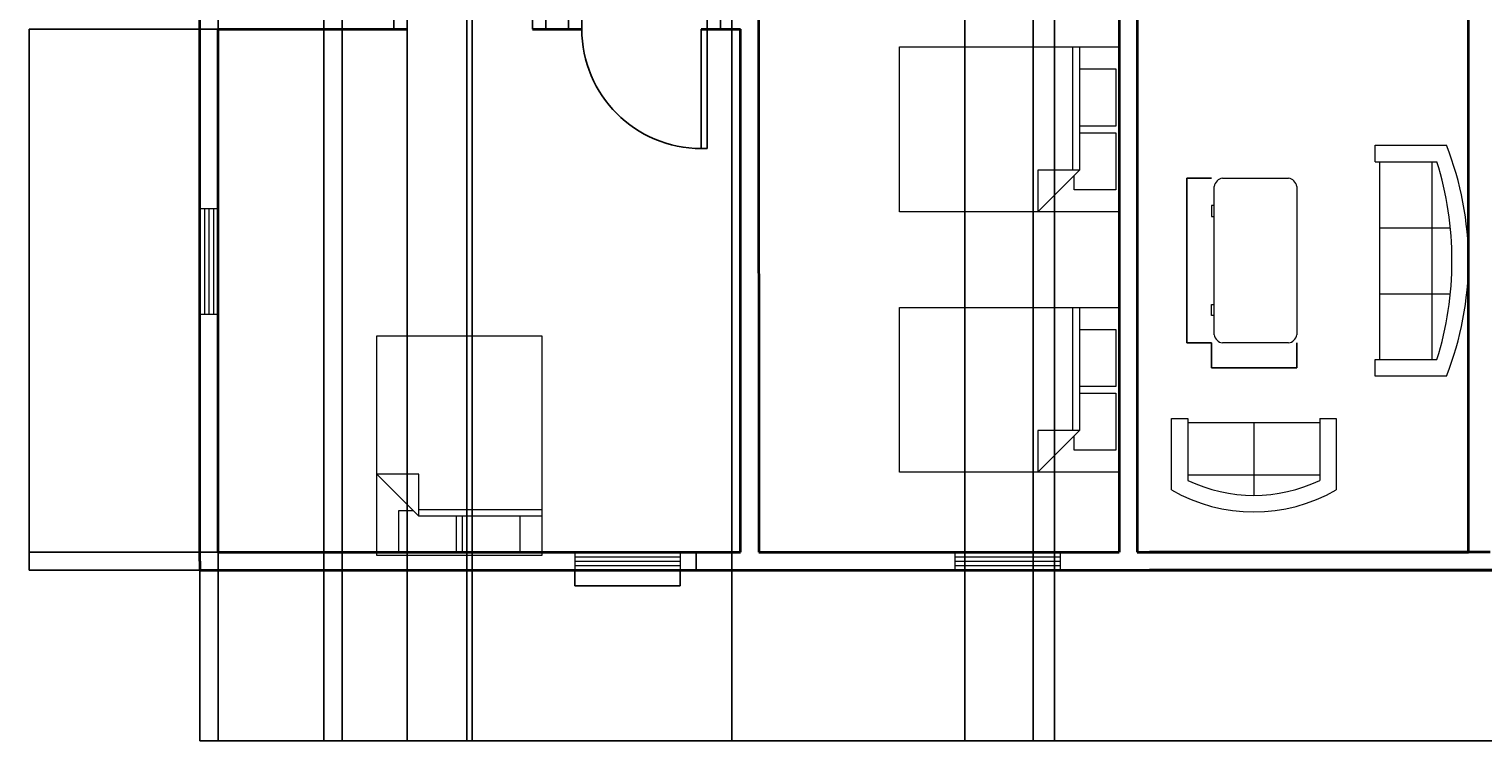
# Model space of a CAD drawing. Units: millimetres. Extents: x 31 to 27050, y -916 to 32407.
# Tile 1 of 7: x 31 to 13474, y -916 to 5664. Entities that reach past the tile are written whole.
import ezdxf

# ---------------------------------------------------------------- set-up
doc = ezdxf.new("R2010")
doc.units = ezdxf.units.MM
for name, color, linetype, lineweight in [('A-ANNO-DIMS', 2, 'Continuous', 18), ('A-DOOR', 3, 'Continuous', 25), ('A-FURN', 8, 'Continuous', 13), ('A-GLAZ', 4, 'Continuous', 18), ('A-WALL', 7, 'Continuous', 35)]:
    doc.layers.add(name, color=color, linetype=linetype, lineweight=lineweight)
doc.styles.get("Standard").update_dxf_attribs({"font": 'arial.ttf'})
doc.dimstyles.get("Standard").update_dxf_attribs({"dimtxt": 0.18, "dimasz": 0.18, "dimexe": 0.18, "dimexo": 0.0625, "dimgap": 0.09, "dimtad": 0, "dimtih": 1, "dimtoh": 1, "dimdec": 4, "dimzin": 0, "dimdsep": 46, "dimtxsty": 'Standard', "dimcen": 0.09, "dimadec": 0, "dimazin": 0, "dimtfac": 1, "dimtdec": 4, "dimtofl": 0, "dimtmove": 0, "dimatfit": 3, "dimfxl": 1, "dimtolj": 1, "dimtzin": 0, "dimarcsym": 0})

# ---------------------------------------------------------------- blocks, each defined once
blk = doc.blocks.new('Sofa - Roundback 7 ft.')
for p, q in [((-12.00002, -32.44210000000393), (-12.00003, -6.597100000003898)), ((11.99996999999999, -32.44210000000393), (11.99997999999999, -6.597100000003898)), ((-36.000027, -34.00000000000395), (-36.000027, -11.46960000000396)), ((-35.999844, -13.38190000000397), (35.99979999999999, -13.38190000000397)), ((35.99997999999999, -34.00000000000395), (35.99997999999999, -11.46960000000396)), ((-36.000027, -32.44210000000393), (35.99997999999999, -32.44210000000393))]:
    blk.add_line(p, q)
for points in [[(-36.000027, -34.00000000000395), (-42.000027, -34.00000000000395), (-42.000027, -8.000000000003944)], [(41.99997999999999, -8.000000000003944), (41.99997999999999, -34.00000000000395), (35.99997999999999, -34.00000000000395)]]:
    blk.add_lwpolyline(points)
for centre, radius, start, end in [((0, -114.2500000000039), 114.2500000000039, 68.43141000000072, 111.5686000000006), ((-1.00000000032e-05, -127.1968000000039), 121.1967999999973, 72.72032999999948, 107.2797000000005)]:
    blk.add_arc(centre, radius, start, end)
blk = doc.blocks.new('Sofa - Roundback Loveseat 5 ft.')
for p, q in [((0, -32.44198000000246), (0, -5.999980000002448)), ((-23.99999999999999, -33.99998000000245), (-23.99999999999999, -11.46958000000243)), ((-23.99979999999998, -13.38178000000245), (23.99986, -13.38178000000245)), ((24.00004000000001, -33.99998000000245), (24.00004000000001, -11.46958000000243)), ((-23.99999999999999, -32.44198000000246), (24.00004000000001, -32.44198000000246))]:
    blk.add_line(p, q)
for points in [[(-23.99999999999999, -33.99998000000245), (-29.99999999999999, -33.99998000000245), (-29.99999999999999, -7.999980000002448)], [(30.00004000000001, -7.999980000002448), (30.00004000000001, -33.99998000000245), (24.00004000000001, -33.99998000000245)]]:
    blk.add_lwpolyline(points)
for centre, radius, start, end in [((0, -60.24998000000245), 60.24998000000245, 60.13715000000122, 119.862800000004), ((0, -61.38438000000245), 55.38444000000723, 64.32083000000306, 115.6791999999996)]:
    blk.add_arc(centre, radius, start, end)
blk = doc.blocks.new('Desk - 30 x 60 in.')
for p, q in [((-26.999995, 0), (26.999995, 0)), ((-29.999995, -27), (-29.999995, -3)), ((29.999995, -3), (29.999995, -27)), ((26.999995, -30), (-26.999995, -30)), ((-20.000005, -30), (-20.000005, -31)), ((-20.000005, -31), (-16.000005, -31)), ((-16.000005, -31), (-16.000005, -30)), ((15.999995, -31), (15.999995, -30)), ((19.999995, -31), (15.999995, -31)), ((19.999995, -30), (19.999995, -31))]:
    blk.add_line(p, q)
for centre, radius, start, end in [((-26.499995, -3.5), 3.535534000004229, 98.1300999999916, 171.8698999999352), ((26.499995, -3.5), 3.535533999997753, 8.130102000022115, 81.8698999999439), ((-26.499995, -26.5), 3.535534000000845, 188.1301000000653, 261.8699000000085), ((26.499995, -26.5), 3.535534000004826, 278.1301000000561, 351.8698999999439)]:
    blk.add_arc(centre, radius, start, end)
blk = doc.blocks.new('Bed - Queen')
for p, q in [((0, -80.00003000000002), (0, 0)), ((0, 0), (59.99998999999999, 0)), ((59.99998999999999, 0), (59.99998999999999, -80.00003000000002)), ((7.99999, -1.200000000000017), (28.79998, -1.200000000000017)), ((7.99999, -14.4), (7.99999, -1.200000000000017)), ((28.79998, -1.200000000000017), (28.79998, -14.4)), ((31.19999, -1.200000000000017), (51.99999000000001, -1.200000000000017)), ((31.19999, -14.4), (31.19999, -1.200000000000017)), ((51.99999000000001, -1.200000000000017), (51.99999000000001, -16.4)), ((0, -14.4), (44.79999999999999, -14.4)), ((59.99998999999999, -29.60000000000001), (44.79999999999999, -14.4)), ((44.79999999999999, -14.4), (44.79999999999999, -29.60000000000001)), ((44.79999999999999, -16.80000000000001), (0, -16.80000000000001)), ((51.99999000000001, -16.4), (46.79936, -16.4)), ((44.79999999999999, -29.60000000000001), (59.99998999999999, -29.60000000000001)), ((59.99998999999999, -80.00003000000002), (0, -80.00003000000002))]:
    blk.add_line(p, q)
blk = doc.blocks.new('Window - Wood Frame 36 in. Wide plan')
for p, q in [((0, 6), (0, 0)), ((36, 6), (36, 0)), ((0, 4.5), (36, 4.5)), ((0, 3), (36, 3)), ((0, 1.5), (36, 1.5))]:
    blk.add_line(p, q)
blk = doc.blocks.new('DOOR-SINGLE-1104')
for p, q in [((56.41678681898429, 1104.337341461596), (-7.18501e-11, 1104.337341461596)), ((-7.18501e-11, 1104.337341461596), (-7.18501e-11, 3.638e-12)), ((56.41678681898429, 7.276e-12), (56.41678681898429, 1104.337341461596)), ((-1226.913698425656, -163.8831223050438), (-1226.913698425656, 3.638e-12)), ((-1104.337341461589, 3.638e-12), (-1226.913698425656, 7.276e-12)), ((-1104.337341461589, 3.638e-12), (-1104.337341461589, -163.8831223050438)), ((-7.18501e-11, 3.638e-12), (56.41678681898429, 7.276e-12)), ((56.41678681898429, -163.8831223050438), (56.41678681898429, 3.638e-12)), ((56.41678681898429, 3.638e-12), (178.9931437830519, 3.638e-12)), ((178.9931437830519, 3.638e-12), (178.9931437830519, -163.8831223050438)), ((-1104.337341461589, -163.8831223050438), (-1226.913698425656, -163.8831223050438)), ((178.9931437830519, -163.8831223050438), (56.41678681898429, -163.8831223050438))]:
    blk.add_line(p, q)
blk.add_arc((0, 3.638e-12), 1104.337341461589, 90, 180)
blk = doc.blocks.new('*D20')
at = {"layer": 'A-ANNO-DIMS', "color": 0, "lineweight": -2, "transparency": 16777216}
for p, q in [((5076.661328165442, 664.7949646643646), (5076.661328165442, 518.2710500577334)), ((6052.70409220965, 664.7949646643646), (6052.70409220965, 518.2710500577334)), ((5076.841328165443, 518.4510500577334), (5563.054422329429, 518.4510500577334)), ((6052.52409220965, 518.4510500577334), (5566.310998045663, 518.4510500577334))]:
    blk.add_line(p, q, dxfattribs=at)
at = {"layer": 'A-ANNO-DIMS', "color": 0, "transparency": 16777216}
for points in [[(5076.841328165443, 518.4810500577335), (5076.841328165443, 518.4210500577335), (5076.661328165442, 518.4510500577334)], [(6052.52409220965, 518.4810500577335), (6052.52409220965, 518.4210500577335), (6052.70409220965, 518.4510500577334)]]:
    blk.add_solid(points, dxfattribs=at)
at = {"layer": 'Defpoints', "color": 0, "transparency": 16777216}
for p in [(5076.661328165442, 664.8574646643647), (6052.70409220965, 664.8574646643647), (6052.70409220965, 518.4510500577334)]:
    blk.add_point(p, dxfattribs=at)
at = {"layer": 'A-ANNO-DIMS', "color": 0, "transparency": 16777216, "insert": (5564.682710187546, 518.4510500577334), "char_height": 0.18, "attachment_point": 5}
blk.add_mtext('\\A1;WOOD WINDOW 976 TYP.', dxfattribs=at)
blk = doc.blocks.new('*D21')
at = {"layer": 'A-ANNO-DIMS', "color": 0, "lineweight": -2, "transparency": 16777216}
for p, q in [((6052.766592209652, 827.531258671733), (6199.290506816289, 827.531258671733)), ((6199.110506816289, 827.351258671733), (6199.110506816289, 746.3763261973802)), ((6199.110506816289, 665.0374646643648), (6199.110506816289, 746.0123971387173)), ((6052.766592209652, 664.8574646643648), (6199.290506816289, 664.8574646643648))]:
    blk.add_line(p, q, dxfattribs=at)
at = {"layer": 'A-ANNO-DIMS', "color": 0, "transparency": 16777216}
for points in [[(6199.080506816289, 827.351258671733), (6199.140506816288, 827.351258671733), (6199.110506816289, 827.531258671733)], [(6199.080506816289, 665.0374646643648), (6199.140506816288, 665.0374646643648), (6199.110506816289, 664.8574646643648)]]:
    blk.add_solid(points, dxfattribs=at)
at = {"layer": 'Defpoints', "color": 0, "transparency": 16777216}
for p in [(6052.704092209652, 827.531258671733), (6199.110506816289, 827.531258671733), (6052.704092209652, 664.8574646643648)]:
    blk.add_point(p, dxfattribs=at)
at = {"layer": 'A-ANNO-DIMS', "color": 0, "transparency": 16777216, "insert": (6199.110506816287, 746.194361668047), "char_height": 0.18, "attachment_point": 5}
blk.add_mtext('\\A1;163 TYP.', dxfattribs=at)
blk = doc.blocks.new('*D38')
at = {"layer": 'A-ANNO-DIMS', "color": 0, "lineweight": -2, "transparency": 16777216}
for p, q in [((10964.92577730674, 4286.348550041928), (10736.20831454058, 4286.348550041928)), ((10736.38831454058, 4286.168550041928), (10736.38831454058, 3524.531743731799)), ((10736.38831454058, 2762.528798267508), (10736.38831454058, 3524.165604577638)), ((10964.92577730674, 2762.348798267508), (10736.20831454058, 2762.348798267508))]:
    blk.add_line(p, q, dxfattribs=at)
at = {"layer": 'A-ANNO-DIMS', "color": 0, "transparency": 16777216}
for points in [[(10736.35831454058, 4286.168550041928), (10736.41831454058, 4286.168550041928), (10736.38831454058, 4286.348550041928)], [(10736.35831454058, 2762.528798267508), (10736.41831454058, 2762.528798267508), (10736.38831454058, 2762.348798267508)]]:
    blk.add_solid(points, dxfattribs=at)
at = {"layer": 'Defpoints', "color": 0, "transparency": 16777216}
for p in [(10964.98827730674, 4286.348550041928), (10736.38831454058, 2762.348798267508), (10964.98827730674, 2762.348798267508)]:
    blk.add_point(p, dxfattribs=at)
at = {"layer": 'A-ANNO-DIMS', "color": 0, "transparency": 16777216, "insert": (10736.38831454058, 3524.348674154714), "char_height": 0.18, "attachment_point": 5}
blk.add_mtext('\\A1;DESK 1524 TYP.', dxfattribs=at)
blk = doc.blocks.new('*D39')
at = {"layer": 'A-ANNO-DIMS', "color": 0, "lineweight": -2, "transparency": 16777216}
for p, q in [((10964.98827730674, 2762.286298267507), (10964.98827730674, 2533.568835501344)), ((11752.38828019396, 2762.286298267507), (11752.38828019396, 2533.568835501344)), ((10965.16827730674, 2533.748835501344), (11358.09100044202, 2533.748835501344)), ((11752.20828019396, 2533.748835501344), (11359.28555705867, 2533.748835501344))]:
    blk.add_line(p, q, dxfattribs=at)
at = {"layer": 'A-ANNO-DIMS', "color": 0, "transparency": 16777216}
for points in [[(10965.16827730674, 2533.778835501344), (10965.16827730674, 2533.718835501344), (10964.98827730674, 2533.748835501344)], [(11752.20828019396, 2533.778835501344), (11752.20828019396, 2533.718835501344), (11752.38828019396, 2533.748835501344)]]:
    blk.add_solid(points, dxfattribs=at)
at = {"layer": 'Defpoints', "color": 0, "transparency": 16777216}
for p in [(10964.98827730674, 2762.348798267507), (11752.38828019396, 2762.348798267507), (11752.38828019396, 2533.748835501344)]:
    blk.add_point(p, dxfattribs=at)
at = {"layer": 'A-ANNO-DIMS', "color": 0, "transparency": 16777216, "insert": (11358.68827875035, 2533.748835501344), "char_height": 0.18, "attachment_point": 5}
blk.add_mtext('\\A1;787 TYP.', dxfattribs=at)
blk = doc.blocks.new('*D46')
at = {"layer": 'A-ANNO-DIMS', "color": 0, "lineweight": -2, "transparency": 16777216}
for p, q in [((1610.021997, 663.585636), (1610.021997, -915.531864)), ((25471.148668, 663.585636), (25471.148668, -915.531864)), ((1610.201997, -915.3518639999999), (13540.17247438267, -915.3518639999999)), ((25470.968668, -915.3518639999999), (13540.99819061733, -915.3518639999999))]:
    blk.add_line(p, q, dxfattribs=at)
at = {"layer": 'A-ANNO-DIMS', "color": 0, "transparency": 16777216}
for points in [[(1610.201997, -915.321864), (1610.201997, -915.381864), (1610.021997, -915.3518639999999)], [(25470.968668, -915.321864), (25470.968668, -915.381864), (25471.148668, -915.3518639999999)]]:
    blk.add_solid(points, dxfattribs=at)
at = {"layer": 'Defpoints', "color": 0, "transparency": 16777216}
for p in [(1610.021997, 663.648136), (25471.148668, 663.648136), (25471.148668, -915.3518639999999)]:
    blk.add_point(p, dxfattribs=at)
at = {"layer": 'A-ANNO-DIMS', "color": 0, "transparency": 16777216, "insert": (13540.5853325, -915.3518639999999), "char_height": 0.18, "attachment_point": 5}
blk.add_mtext('\\A1;23861', dxfattribs=at)
blk = doc.blocks.new('*D59')
at = {"layer": 'A-ANNO-DIMS', "color": 0, "lineweight": -2, "transparency": 16777216}
for p, q in [((1778.310148000001, 5663.648136000002), (30.84199699999942, 5663.648136000002)), ((31.02199699999949, 5663.468136000002), (31.02199700000003, 3245.771662029333)), ((31.02199700000057, 827.7112590000002), (31.02199700000003, 3245.407732970669)), ((1778.310148000001, 827.5312590000003), (30.8419970000005, 827.5312590000002))]:
    blk.add_line(p, q, dxfattribs=at)
at = {"layer": 'A-ANNO-DIMS', "color": 0, "transparency": 16777216}
for points in [[(30.99199699999949, 5663.468136000002), (31.05199699999949, 5663.468136000002), (31.02199699999949, 5663.648136000002)], [(30.99199700000057, 827.7112590000002), (31.05199700000057, 827.7112590000002), (31.02199700000057, 827.5312590000002)]]:
    blk.add_solid(points, dxfattribs=at)
at = {"layer": 'Defpoints', "color": 0, "transparency": 16777216}
for p in [(31.02199699999949, 5663.648136000002), (1778.372648000001, 5663.648136000002), (1778.372648000001, 827.5312590000003)]:
    blk.add_point(p, dxfattribs=at)
at = {"layer": 'A-ANNO-DIMS', "color": 0, "transparency": 16777216, "insert": (31.02199700000094, 3245.5896975), "char_height": 0.18, "attachment_point": 5}
blk.add_mtext('\\A1;4836', dxfattribs=at)
blk = doc.blocks.new('*D69')
at = {"layer": 'A-ANNO-DIMS', "color": 0, "lineweight": -2, "transparency": 16777216}
for p, q in [((2757.340836, 14467.362437), (2757.340835999999, -915.5318640000004)), ((4128.594056999999, 14467.362437), (4128.594056999999, -915.5318640000004)), ((2757.520835999999, -915.3518639999999), (3442.512289610504, -915.3518639999999)), ((4128.414056999999, -915.3518639999999), (3443.422603389495, -915.3518639999999))]:
    blk.add_line(p, q, dxfattribs=at)
at = {"layer": 'A-ANNO-DIMS', "color": 0, "transparency": 16777216}
for points in [[(2757.520835999999, -915.321864), (2757.520835999999, -915.381864), (2757.340835999999, -915.3518639999999)], [(4128.414056999999, -915.321864), (4128.414056999999, -915.381864), (4128.594056999999, -915.3518639999999)]]:
    blk.add_solid(points, dxfattribs=at)
at = {"layer": 'Defpoints', "color": 0, "transparency": 16777216}
for p in [(2757.340836, 14467.424937), (4128.594056999999, 14467.424937), (4128.594056999999, -915.3518639999999)]:
    blk.add_point(p, dxfattribs=at)
at = {"layer": 'A-ANNO-DIMS', "color": 0, "transparency": 16777216, "insert": (3442.967446499999, -915.3518639999999), "char_height": 0.18, "attachment_point": 5}
blk.add_mtext('\\A1;1371.3', dxfattribs=at)
blk = doc.blocks.new('*D70')
at = {"layer": 'A-ANNO-DIMS', "color": 0, "lineweight": -2, "transparency": 16777216}
for p, q in [((4128.594056999999, 14467.362437), (4128.594056999999, -915.5318640000004)), ((6528.594057000001, 14467.362437), (6528.594056999999, -915.5318640000004)), ((4128.774057, -915.3518639999999), (5328.234056999999, -915.3518639999999)), ((6528.414056999999, -915.3518639999999), (5328.954056999999, -915.3518639999999))]:
    blk.add_line(p, q, dxfattribs=at)
at = {"layer": 'A-ANNO-DIMS', "color": 0, "transparency": 16777216}
for points in [[(4128.774057, -915.321864), (4128.774057, -915.381864), (4128.594056999999, -915.3518639999999)], [(6528.414056999999, -915.321864), (6528.414056999999, -915.381864), (6528.594056999999, -915.3518639999999)]]:
    blk.add_solid(points, dxfattribs=at)
at = {"layer": 'Defpoints', "color": 0, "transparency": 16777216}
for p in [(4128.594056999999, 14467.424937), (6528.594057000001, 14467.424937), (6528.594056999999, -915.3518639999999)]:
    blk.add_point(p, dxfattribs=at)
at = {"layer": 'A-ANNO-DIMS', "color": 0, "transparency": 16777216, "insert": (5328.594057, -915.3518639999999), "char_height": 0.18, "attachment_point": 5}
blk.add_mtext('\\A1;2400', dxfattribs=at)
blk = doc.blocks.new('*D74')
at = {"layer": 'A-ANNO-DIMS', "color": 0, "lineweight": -2, "transparency": 16777216}
for p, q in [((8684.522829, 19025.373224), (8684.522828999998, -915.5318640000004)), ((9513.331407, 19025.373224), (9513.331407, -915.5318640000004)), ((8684.702829, -915.3518639999999), (9098.533107085947, -915.3518639999999)), ((9513.151406999998, -915.3518639999999), (9099.321128914047, -915.3518639999999))]:
    blk.add_line(p, q, dxfattribs=at)
at = {"layer": 'A-ANNO-DIMS', "color": 0, "transparency": 16777216}
for points in [[(8684.702829, -915.321864), (8684.702829, -915.381864), (8684.522828999998, -915.3518639999999)], [(9513.151406999998, -915.321864), (9513.151406999998, -915.381864), (9513.331407, -915.3518639999999)]]:
    blk.add_solid(points, dxfattribs=at)
at = {"layer": 'Defpoints', "color": 0, "transparency": 16777216}
for p in [(8684.522829, 19025.435724), (9513.331407, 19025.435724), (8684.522828999998, -915.3518639999999)]:
    blk.add_point(p, dxfattribs=at)
at = {"layer": 'A-ANNO-DIMS', "color": 0, "transparency": 16777216, "insert": (9098.927117999998, -915.3518639999999), "char_height": 0.18, "attachment_point": 5}
blk.add_mtext('\\A1;828.8', dxfattribs=at)
blk = doc.blocks.new('*D75')
at = {"layer": 'A-ANNO-DIMS', "color": 0, "lineweight": -2, "transparency": 16777216}
for p, q in [((9315.42813, 12465.681171), (9315.42813, -915.5318640000004)), ((9513.331407, 12465.681171), (9513.331407, -915.5318640000004)), ((9315.60813, -915.3518639999999), (9413.994352401773, -915.3518639999999)), ((9513.151407, -915.3518639999999), (9414.765184598225, -915.3518639999999))]:
    blk.add_line(p, q, dxfattribs=at)
at = {"layer": 'A-ANNO-DIMS', "color": 0, "transparency": 16777216}
for points in [[(9315.60813, -915.321864), (9315.60813, -915.381864), (9315.42813, -915.3518639999999)], [(9513.151407, -915.321864), (9513.151407, -915.381864), (9513.331407, -915.3518639999999)]]:
    blk.add_solid(points, dxfattribs=at)
at = {"layer": 'Defpoints', "color": 0, "transparency": 16777216}
for p in [(9315.42813, 12465.743671), (9513.331407, 12465.743671), (9513.331407, -915.3518639999999)]:
    blk.add_point(p, dxfattribs=at)
at = {"layer": 'A-ANNO-DIMS', "color": 0, "transparency": 16777216, "insert": (9414.379768499999, -915.3518639999999), "char_height": 0.18, "attachment_point": 5}
blk.add_mtext('\\A1;197.9', dxfattribs=at)
blk = doc.blocks.new('*D88')
at = {"layer": 'A-ANNO-DIMS', "color": 0, "lineweight": -2, "transparency": 16777216}
for p, q in [((1778.310148000001, 827.5312590000003), (30.84199700000004, 827.5312590000002)), ((31.02199700000001, 827.3512590000003), (31.02199700000003, 745.7716620293315)), ((31.02199700000005, 663.8281359999999), (31.02199700000003, 745.4077329706685)), ((1609.959497000001, 663.6481360000002), (30.84199700000008, 663.648136))]:
    blk.add_line(p, q, dxfattribs=at)
at = {"layer": 'A-ANNO-DIMS', "color": 0, "transparency": 16777216}
for points in [[(30.99199700000001, 827.3512590000003), (31.05199700000001, 827.3512590000003), (31.02199700000001, 827.5312590000002)], [(30.99199700000005, 663.8281359999999), (31.05199700000005, 663.8281359999999), (31.02199700000005, 663.648136)]]:
    blk.add_solid(points, dxfattribs=at)
at = {"layer": 'Defpoints', "color": 0, "transparency": 16777216}
for p in [(31.02199700000001, 827.5312590000002), (1778.372648000001, 827.5312590000003), (1610.021997000001, 663.6481360000002)]:
    blk.add_point(p, dxfattribs=at)
at = {"layer": 'A-ANNO-DIMS', "color": 0, "transparency": 16777216, "insert": (31.02199700000023, 745.5896974999999), "char_height": 0.18, "attachment_point": 5}
blk.add_mtext('\\A1;163.88', dxfattribs=at)
blk = doc.blocks.new('*D92')
at = {"layer": 'A-ANNO-DIMS', "color": 0, "lineweight": -2, "transparency": 16777216}
for p, q in [((1778.372648, 5827.468759000001), (1778.372647999999, -915.5318640000004)), ((3525.344535, 5827.468759000001), (3525.344535, -915.5318640000004)), ((1778.552647999999, -915.3518639999999), (2651.508291363575, -915.3518639999999)), ((3525.164535, -915.3518639999999), (2652.208891636425, -915.3518639999999))]:
    blk.add_line(p, q, dxfattribs=at)
at = {"layer": 'A-ANNO-DIMS', "color": 0, "transparency": 16777216}
for points in [[(1778.552647999999, -915.321864), (1778.552647999999, -915.381864), (1778.372647999999, -915.3518639999999)], [(3525.164535, -915.321864), (3525.164535, -915.381864), (3525.344535, -915.3518639999999)]]:
    blk.add_solid(points, dxfattribs=at)
at = {"layer": 'Defpoints', "color": 0, "transparency": 16777216}
for p in [(1778.372648, 5827.531259), (3525.344535, 5827.531259), (3525.344535, -915.3518639999999)]:
    blk.add_point(p, dxfattribs=at)
at = {"layer": 'A-ANNO-DIMS', "color": 0, "transparency": 16777216, "insert": (2651.8585915, -915.3518639999999), "char_height": 0.18, "attachment_point": 5}
blk.add_mtext('\\A1;1747', dxfattribs=at)
blk = doc.blocks.new('*D93')
at = {"layer": 'A-ANNO-DIMS', "color": 0, "lineweight": -2, "transparency": 16777216}
for p, q in [((2925.691486, 14303.479314), (2925.691486, -915.5318640000004)), ((4078.94748, 14303.479314), (4078.947479999999, -915.5318640000004)), ((2925.871485999999, -915.3518639999999), (3501.864326110504, -915.3518639999999)), ((4078.767479999998, -915.3518639999999), (3502.774639889495, -915.3518639999999))]:
    blk.add_line(p, q, dxfattribs=at)
at = {"layer": 'A-ANNO-DIMS', "color": 0, "transparency": 16777216}
for points in [[(2925.871485999999, -915.321864), (2925.871485999999, -915.381864), (2925.691486, -915.3518639999999)], [(4078.767479999998, -915.321864), (4078.767479999998, -915.381864), (4078.947479999999, -915.3518639999999)]]:
    blk.add_solid(points, dxfattribs=at)
at = {"layer": 'Defpoints', "color": 0, "transparency": 16777216}
for p in [(2925.691486, 14303.541814), (4078.94748, 14303.541814), (4078.947479999999, -915.3518639999999)]:
    blk.add_point(p, dxfattribs=at)
at = {"layer": 'A-ANNO-DIMS', "color": 0, "transparency": 16777216, "insert": (3502.319482999999, -915.3518639999999), "char_height": 0.18, "attachment_point": 5}
blk.add_mtext('\\A1;1153.3', dxfattribs=at)

msp = doc.modelspace()

# ---------------------------------------------------------------- linework, layer by layer
at = {"layer": 'A-WALL'}
for p, q in [((10278.37264782516, 12938.12750679554), (10278.37264782516, 827.5312586717337)), ((13340.58533261045, 827.5312586717337), (13340.58533261045, 12938.12750679554)), ((1610.021997114469, 744.3803777755929), (1610.021997114469, 12465.74367114627)), ((10110.02199711447, 8571.211098631777), (10110.02199711447, 827.5312586717337)), ((6773.905119419524, 7115.269042771405), (6778.372647825162, 827.5312586717337)), ((1778.372647825163, 5663.648136366682), (3525.344534980938, 5663.648136366682)), ((1778.372647825163, 827.5312586717337), (1778.372647825163, 5663.648136366682)), ((4686.09866326151, 5663.648136366682), (5141.43722246237, 5663.648136366682)), ((6245.774563923887, 5663.648136366682), (6610.021997114469, 5663.648136366682)), ((6610.021997114469, 827.5312586717337), (6610.021997114469, 5663.648136366681)), ((1778.372647825163, 827.5312586717337), (6610.021997114471, 827.5312586717337)), ((6778.372647825162, 827.5312586717337), (10110.02199711447, 827.5312586717337)), ((10278.37264782516, 827.5312586717337), (13340.58533261045, 827.5312586717336)), ((13540.58533261045, 827.5312586717337), (10390.58533261045, 827.5312586717337)), ((1610.021997114469, 744.3803777755929), (1610.021997114469, 663.6481363666826)), ((1610.021997114469, 663.6481363666826), (1690.58533261045, 663.6481363666826)), ((1690.58533261045, 663.6481363666826), (10190.58533261045, 663.6481363666826)), ((10190.58533261045, 663.6481363666826), (16690.58533261045, 663.6481363666826)), ((16890.58533261045, 663.6481363666826), (10390.58533261045, 663.6481363666826))]:
    msp.add_line(p, q, dxfattribs=at)

# ---------------------------------------------------------------- block references
at = {"layer": 'A-DOOR'}
msp.add_blockref('DOOR-SINGLE-1104', (4629.681876442521, 5827.531258671719), dxfattribs=at)
at = {"layer": 'A-DOOR', "extrusion": (0, 0, -1), "zscale": -1, "rotation": 180}
msp.add_blockref('DOOR-SINGLE-1104', (-6245.774563923957, 5663.648136366701), dxfattribs=at)
at = {"layer": 'A-FURN', "xscale": 25.4, "yscale": 25.4, "zscale": 25.4}
for name, p, rotation in [('Bed - Queen', (10110.02199711446, 5498.496041437785), 270), ('Sofa - Roundback 7 ft.', (13340.58533261045, 3522.960061555132), 270), ('Desk - 30 x 60 in.', (11752.38827730674, 3524.348674154725), 270), ('Bed - Queen', (10110.02199711446, 3091.368000807226), 270), ('Bed - Queen', (4771.30648783152, 797.0512586717331), 180), ('Sofa - Roundback Loveseat 5 ft.', (11356.03248513326, 1201.42641839608), 180)]:
    msp.add_blockref(name, p, dxfattribs=dict(at, rotation=rotation))
at = {"layer": 'A-GLAZ', "xscale": 27.11229900122799, "yscale": 27.11229900122799, "zscale": 27.11229900122799, "rotation": 90}
msp.add_blockref('Window - Wood Frame 36 in. Wide plan', (1778.372647825162, 3030.203903365821), dxfattribs=at)
at = {"layer": 'A-GLAZ', "xscale": 27.11229900122799, "yscale": 27.11229900122799, "zscale": 27.11229900122799}
for p in [(5076.661328165443, 664.8574646643647), (8590.415340123465, 664.8574646643647)]:
    msp.add_blockref('Window - Wood Frame 36 in. Wide plan', p, dxfattribs=at)

# ---------------------------------------------------------------- dimensions: what is measured, and where the dimension line sits
at = {"layer": 'A-ANNO-DIMS'}
for base, p1, p2, override, picture, middle in [((8684.522828999998, -915.3518639999999), (9513.331407, 19025.435724), (8684.522829, 19025.435724), {"dimdec": 1, "dimlfac": 1, "dimrnd": 0, "dimzin": 0, "dimdsep": 46, "dimlunit": 2}, '*D74', (9098.927117999998, -915.3518639999999)), ((4128.594056999999, -915.3518639999999), (2757.340836, 14467.424937), (4128.594056999999, 14467.424937), {"dimdec": 1, "dimlfac": 1, "dimrnd": 0, "dimzin": 0, "dimdsep": 46, "dimlunit": 2}, '*D69', (3442.967446499999, -915.3518639999999)), ((6528.594056999999, -915.3518639999999), (4128.594056999999, 14467.424937), (6528.594057000001, 14467.424937), {"dimdec": 0, "dimlfac": 1, "dimrnd": 0, "dimzin": 0, "dimdsep": 46, "dimlunit": 2}, '*D70', (5328.594057, -915.3518639999999)), ((4078.947479999999, -915.3518639999999), (2925.691486, 14303.541814), (4078.94748, 14303.541814), {"dimdec": 1, "dimlfac": 1, "dimrnd": 0, "dimzin": 0, "dimdsep": 46, "dimlunit": 2}, '*D93', (3502.319482999999, -915.3518639999999)), ((9513.331407, -915.3518639999999), (9315.42813, 12465.743671), (9513.331407, 12465.743671), {"dimdec": 1, "dimlfac": 1, "dimrnd": 0, "dimzin": 0, "dimdsep": 46, "dimlunit": 2}, '*D75', (9414.379768499999, -915.3518639999999)), ((3525.344535, -915.3518639999999), (1778.372648, 5827.531259), (3525.344535, 5827.531259), {"dimdec": 0, "dimlfac": 1, "dimrnd": 0, "dimzin": 0, "dimdsep": 46, "dimlunit": 2}, '*D92', (2651.8585915, -915.3518639999999)), ((25471.148668, -915.3518639999999), (1610.021997, 663.648136), (25471.148668, 663.648136), {"dimdec": 0, "dimlfac": 1, "dimrnd": 0, "dimzin": 0, "dimdsep": 46, "dimlunit": 2}, '*D46', (13540.5853325, -915.3518639999999))]:
    dim = msp.add_linear_dim(base=base, p1=p1, p2=p2, dimstyle='Standard', override=override, dxfattribs=at)
    dim.commit()
    dim.dimension.update_dxf_attribs({"geometry": picture, "text_midpoint": middle})
for base, p1, p2, override, picture, middle in [((31.02199699999949, 5663.648136000002), (1778.372648, 827.531259), (1778.372648, 5663.648135999999), {"dimdec": 0, "dimlfac": 1, "dimrnd": 0, "dimzin": 0, "dimdsep": 46, "dimlunit": 2}, '*D59', (31.02199700000094, 3245.5896975)), ((31.02199700000001, 827.5312590000002), (1610.021997, 663.648136), (1778.372648, 827.531259), {"dimdec": 2, "dimlfac": 1, "dimrnd": 0, "dimzin": 0, "dimdsep": 46, "dimlunit": 2}, '*D88', (31.02199700000023, 745.5896974999999))]:
    dim = msp.add_linear_dim(base=base, p1=p1, p2=p2, angle=90, dimstyle='Standard', override=override, dxfattribs=at)
    dim.commit()
    dim.dimension.update_dxf_attribs({"geometry": picture, "text_midpoint": middle})
for base, p1, p2, angle, text, picture, middle in [((10736.38831454058, 2762.348798267508), (10964.98827730674, 4286.348550041926), (10964.98827730674, 2762.348798267507), 270, 'DESK <> TYP.', '*D38', (10736.38831454058, 3524.348674154714)), ((6199.110506816289, 827.531258671733), (6052.70409220965, 664.8574646643647), (6052.70409220965, 827.5312586717324), 90, '<> TYP.', '*D21', (6199.110506816287, 746.194361668047))]:
    dim = msp.add_linear_dim(base=base, p1=p1, p2=p2, angle=angle, text=text, dimstyle='Standard', override={"dimdec": 0, "dimlfac": 1, "dimrnd": 0, "dimzin": 0, "dimdsep": 46, "dimlunit": 2}, dxfattribs=at)
    dim.commit()
    dim.dimension.update_dxf_attribs({"geometry": picture, "text_midpoint": middle})
for base, p1, p2, text, picture, middle in [((11752.38828019396, 2533.748835501344), (10964.98827730674, 2762.348798267507), (11752.38828019396, 2762.348798267507), '<> TYP.', '*D39', (11358.68827875035, 2533.748835501344)), ((6052.70409220965, 518.4510500577334), (5076.661328165442, 664.8574646643647), (6052.70409220965, 664.8574646643647), 'WOOD WINDOW <> TYP.', '*D20', (5564.682710187546, 518.4510500577334))]:
    dim = msp.add_linear_dim(base=base, p1=p1, p2=p2, text=text, dimstyle='Standard', override={"dimdec": 0, "dimlfac": 1, "dimrnd": 0, "dimzin": 0, "dimdsep": 46, "dimlunit": 2}, dxfattribs=at)
    dim.commit()
    dim.dimension.update_dxf_attribs({"geometry": picture, "text_midpoint": middle})

doc.saveas('drawing.dxf')
